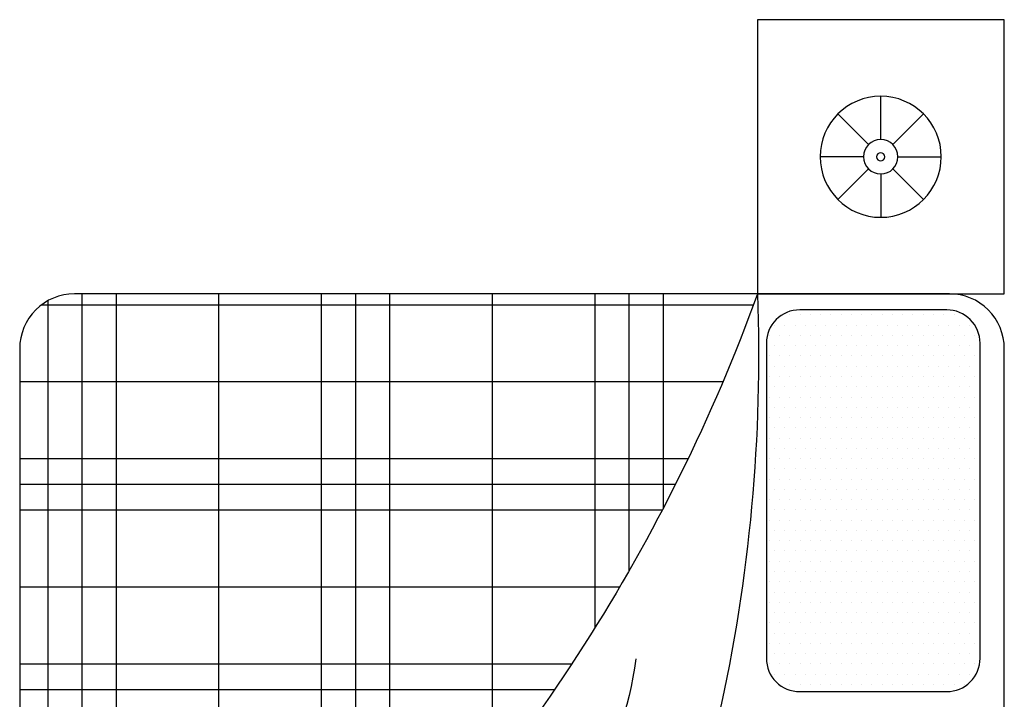
# Model space of a CAD drawing. Units: inches. Extents: x 528 to 2520, y -151 to 1354.
# Tile 12 of 41: x 814 to 869, y 1189 to 1227. Entities that reach past the tile are written whole.
import ezdxf

# ---------------------------------------------------------------- set-up
doc = ezdxf.new("R2010")
doc.units = ezdxf.units.IN
doc.header["$MEASUREMENT"] = 0
doc.layers.add('A-FURN', color=8, linetype='Continuous', lineweight=18)
doc.layers.add('BLOCK', color=6, linetype='Continuous')

# ---------------------------------------------------------------- blocks, each defined once
blk = doc.blocks.new('*X15')
at = {"color": 0}
for p, q in [((276.598, 451.25), (280.51, 451.25)), ((275.455, 450.625), (280.51, 450.625)), ((274.411, 450), (280.51, 450)), ((265.51, 448.125), (267.634, 448.125)), ((271.723, 448.125), (280.51, 448.125)), ((265.51, 446.25), (268.465, 446.25)), ((269.519, 446.25), (280.51, 446.25)), ((265.51, 445.625), (268.531, 445.625)), ((268.866, 445.625), (280.51, 445.625)), ((265.51, 445), (280.51, 445)), ((265.51, 443.125), (280.51, 443.125)), ((265.51, 441.25), (280.51, 441.25)), ((265.51, 440.625), (280.51, 440.625)), ((265.634, 440), (280.386, 440))]:
    blk.add_line(p, q, dxfattribs=at)
blk = doc.blocks.new('*X16')
at = {"color": 0}
for p, q in [((280.312, 439.886), (280.312, 452.896)), ((278.906, 439.482), (278.906, 452.338)), ((277.5, 439.482), (277.5, 451.702)), ((277.031, 439.482), (277.031, 451.471)), ((276.562, 439.482), (276.562, 451.231)), ((275.156, 439.482), (275.156, 450.451)), ((265.781, 439.797), (265.781, 449.511)), ((273.75, 439.482), (273.75, 449.576)), ((266.25, 439.517), (266.25, 449.296)), ((273.281, 439.482), (273.281, 449.261)), ((272.812, 439.482), (272.812, 448.934)), ((267.656, 439.482), (267.656, 448.095)), ((271.406, 439.482), (271.406, 447.876)), ((270, 439.482), (270, 446.689)), ((269.531, 439.482), (269.531, 446.262)), ((269.062, 439.482), (269.062, 445.817))]:
    blk.add_line(p, q, dxfattribs=at)
blk = doc.blocks.new('*X17')
at = {"color": 0}
for p, q in [((273.9375, 457.03125), (273.9375, 457.03125)), ((274.3125, 457.03125), (274.3125, 457.03125)), ((274.6875, 457.03125), (274.6875, 457.03125)), ((275.0625, 457.03125), (275.0625, 457.03125)), ((275.4375, 457.03125), (275.4375, 457.03125)), ((275.8125, 457.03125), (275.8125, 457.03125)), ((276.1875, 457.03125), (276.1875, 457.03125)), ((276.5625, 457.03125), (276.5625, 457.03125)), ((276.9375, 457.03125), (276.9375, 457.03125)), ((277.3125, 457.03125), (277.3125, 457.03125)), ((277.6875, 457.03125), (277.6875, 457.03125)), ((278.0625, 457.03125), (278.0625, 457.03125)), ((278.4375, 457.03125), (278.4375, 457.03125)), ((278.8125, 457.03125), (278.8125, 457.03125)), ((279.1875, 457.03125), (279.1875, 457.03125)), ((279.5625, 457.03125), (279.5625, 457.03125)), ((273.5625, 456.84375), (273.5625, 456.84375)), ((273.75, 456.9375), (273.75, 456.9375)), ((273.9375, 456.84375), (273.9375, 456.84375)), ((274.125, 456.9375), (274.125, 456.9375)), ((274.3125, 456.84375), (274.3125, 456.84375)), ((274.5, 456.9375), (274.5, 456.9375)), ((274.6875, 456.84375), (274.6875, 456.84375)), ((274.875, 456.9375), (274.875, 456.9375)), ((275.0625, 456.84375), (275.0625, 456.84375)), ((275.25, 456.9375), (275.25, 456.9375)), ((275.4375, 456.84375), (275.4375, 456.84375)), ((275.625, 456.9375), (275.625, 456.9375)), ((275.8125, 456.84375), (275.8125, 456.84375)), ((276, 456.9375), (276, 456.9375)), ((276.1875, 456.84375), (276.1875, 456.84375)), ((276.375, 456.9375), (276.375, 456.9375)), ((276.5625, 456.84375), (276.5625, 456.84375)), ((276.75, 456.9375), (276.75, 456.9375)), ((276.9375, 456.84375), (276.9375, 456.84375)), ((277.125, 456.9375), (277.125, 456.9375)), ((277.3125, 456.84375), (277.3125, 456.84375)), ((277.5, 456.9375), (277.5, 456.9375)), ((277.6875, 456.84375), (277.6875, 456.84375)), ((277.875, 456.9375), (277.875, 456.9375)), ((278.0625, 456.84375), (278.0625, 456.84375)), ((278.25, 456.9375), (278.25, 456.9375)), ((278.4375, 456.84375), (278.4375, 456.84375)), ((278.625, 456.9375), (278.625, 456.9375)), ((278.8125, 456.84375), (278.8125, 456.84375)), ((279, 456.9375), (279, 456.9375)), ((279.1875, 456.84375), (279.1875, 456.84375)), ((279.375, 456.9375), (279.375, 456.9375)), ((279.5625, 456.84375), (279.5625, 456.84375)), ((279.75, 456.9375), (279.75, 456.9375)), ((279.9375, 456.84375), (279.9375, 456.84375)), ((273.375, 456.75), (273.375, 456.75)), ((273.75, 456.75), (273.75, 456.75)), ((274.125, 456.75), (274.125, 456.75)), ((274.5, 456.75), (274.5, 456.75)), ((274.875, 456.75), (274.875, 456.75)), ((275.25, 456.75), (275.25, 456.75)), ((275.625, 456.75), (275.625, 456.75)), ((276, 456.75), (276, 456.75)), ((276.375, 456.75), (276.375, 456.75)), ((276.75, 456.75), (276.75, 456.75)), ((277.125, 456.75), (277.125, 456.75)), ((277.5, 456.75), (277.5, 456.75)), ((277.875, 456.75), (277.875, 456.75)), ((278.25, 456.75), (278.25, 456.75)), ((278.625, 456.75), (278.625, 456.75)), ((279, 456.75), (279, 456.75)), ((279.375, 456.75), (279.375, 456.75)), ((279.75, 456.75), (279.75, 456.75)), ((280.125, 456.75), (280.125, 456.75)), ((273.375, 456.5625), (273.375, 456.5625)), ((273.5625, 456.65625), (273.5625, 456.65625)), ((273.75, 456.5625), (273.75, 456.5625)), ((273.9375, 456.65625), (273.9375, 456.65625)), ((274.125, 456.5625), (274.125, 456.5625)), ((274.3125, 456.65625), (274.3125, 456.65625)), ((274.5, 456.5625), (274.5, 456.5625)), ((274.6875, 456.65625), (274.6875, 456.65625)), ((274.875, 456.5625), (274.875, 456.5625)), ((275.0625, 456.65625), (275.0625, 456.65625)), ((275.25, 456.5625), (275.25, 456.5625)), ((275.4375, 456.65625), (275.4375, 456.65625)), ((275.625, 456.5625), (275.625, 456.5625)), ((275.8125, 456.65625), (275.8125, 456.65625)), ((276, 456.5625), (276, 456.5625)), ((276.1875, 456.65625), (276.1875, 456.65625)), ((276.375, 456.5625), (276.375, 456.5625)), ((276.5625, 456.65625), (276.5625, 456.65625)), ((276.75, 456.5625), (276.75, 456.5625)), ((276.9375, 456.65625), (276.9375, 456.65625)), ((277.125, 456.5625), (277.125, 456.5625)), ((277.3125, 456.65625), (277.3125, 456.65625)), ((277.5, 456.5625), (277.5, 456.5625)), ((277.6875, 456.65625), (277.6875, 456.65625)), ((277.875, 456.5625), (277.875, 456.5625)), ((278.0625, 456.65625), (278.0625, 456.65625)), ((278.25, 456.5625), (278.25, 456.5625)), ((278.4375, 456.65625), (278.4375, 456.65625)), ((278.625, 456.5625), (278.625, 456.5625)), ((278.8125, 456.65625), (278.8125, 456.65625)), ((279, 456.5625), (279, 456.5625)), ((279.1875, 456.65625), (279.1875, 456.65625)), ((279.375, 456.5625), (279.375, 456.5625)), ((279.5625, 456.65625), (279.5625, 456.65625)), ((279.75, 456.5625), (279.75, 456.5625)), ((279.9375, 456.65625), (279.9375, 456.65625)), ((280.125, 456.5625), (280.125, 456.5625)), ((273.375, 456.375), (273.375, 456.375)), ((273.5625, 456.46875), (273.5625, 456.46875)), ((273.75, 456.375), (273.75, 456.375)), ((273.9375, 456.46875), (273.9375, 456.46875)), ((274.125, 456.375), (274.125, 456.375)), ((274.3125, 456.46875), (274.3125, 456.46875)), ((274.5, 456.375), (274.5, 456.375)), ((274.6875, 456.46875), (274.6875, 456.46875)), ((274.875, 456.375), (274.875, 456.375)), ((275.0625, 456.46875), (275.0625, 456.46875)), ((275.25, 456.375), (275.25, 456.375)), ((275.4375, 456.46875), (275.4375, 456.46875)), ((275.625, 456.375), (275.625, 456.375)), ((275.8125, 456.46875), (275.8125, 456.46875)), ((276, 456.375), (276, 456.375)), ((276.1875, 456.46875), (276.1875, 456.46875)), ((276.375, 456.375), (276.375, 456.375)), ((276.5625, 456.46875), (276.5625, 456.46875)), ((276.75, 456.375), (276.75, 456.375)), ((276.9375, 456.46875), (276.9375, 456.46875)), ((277.125, 456.375), (277.125, 456.375)), ((277.3125, 456.46875), (277.3125, 456.46875)), ((277.5, 456.375), (277.5, 456.375)), ((277.6875, 456.46875), (277.6875, 456.46875)), ((277.875, 456.375), (277.875, 456.375)), ((278.0625, 456.46875), (278.0625, 456.46875)), ((278.25, 456.375), (278.25, 456.375)), ((278.4375, 456.46875), (278.4375, 456.46875)), ((278.625, 456.375), (278.625, 456.375)), ((278.8125, 456.46875), (278.8125, 456.46875)), ((279, 456.375), (279, 456.375)), ((279.1875, 456.46875), (279.1875, 456.46875)), ((279.375, 456.375), (279.375, 456.375)), ((279.5625, 456.46875), (279.5625, 456.46875)), ((279.75, 456.375), (279.75, 456.375)), ((279.9375, 456.46875), (279.9375, 456.46875)), ((280.125, 456.375), (280.125, 456.375)), ((273.375, 456.1875), (273.375, 456.1875)), ((273.5625, 456.28125), (273.5625, 456.28125)), ((273.75, 456.1875), (273.75, 456.1875)), ((273.9375, 456.28125), (273.9375, 456.28125)), ((274.125, 456.1875), (274.125, 456.1875)), ((274.3125, 456.28125), (274.3125, 456.28125)), ((274.5, 456.1875), (274.5, 456.1875)), ((274.6875, 456.28125), (274.6875, 456.28125)), ((274.875, 456.1875), (274.875, 456.1875)), ((275.0625, 456.28125), (275.0625, 456.28125)), ((275.25, 456.1875), (275.25, 456.1875)), ((275.4375, 456.28125), (275.4375, 456.28125)), ((275.625, 456.1875), (275.625, 456.1875)), ((275.8125, 456.28125), (275.8125, 456.28125)), ((276, 456.1875), (276, 456.1875)), ((276.1875, 456.28125), (276.1875, 456.28125)), ((276.375, 456.1875), (276.375, 456.1875)), ((276.5625, 456.28125), (276.5625, 456.28125)), ((276.75, 456.1875), (276.75, 456.1875)), ((276.9375, 456.28125), (276.9375, 456.28125)), ((277.125, 456.1875), (277.125, 456.1875)), ((277.3125, 456.28125), (277.3125, 456.28125)), ((277.5, 456.1875), (277.5, 456.1875)), ((277.6875, 456.28125), (277.6875, 456.28125)), ((277.875, 456.1875), (277.875, 456.1875)), ((278.0625, 456.28125), (278.0625, 456.28125)), ((278.25, 456.1875), (278.25, 456.1875)), ((278.4375, 456.28125), (278.4375, 456.28125)), ((278.625, 456.1875), (278.625, 456.1875)), ((278.8125, 456.28125), (278.8125, 456.28125)), ((279, 456.1875), (279, 456.1875)), ((279.1875, 456.28125), (279.1875, 456.28125)), ((279.375, 456.1875), (279.375, 456.1875)), ((279.5625, 456.28125), (279.5625, 456.28125)), ((279.75, 456.1875), (279.75, 456.1875)), ((279.9375, 456.28125), (279.9375, 456.28125)), ((280.125, 456.1875), (280.125, 456.1875)), ((273.375, 456), (273.375, 456)), ((273.5625, 456.09375), (273.5625, 456.09375)), ((273.75, 456), (273.75, 456)), ((273.9375, 456.09375), (273.9375, 456.09375)), ((274.125, 456), (274.125, 456)), ((274.3125, 456.09375), (274.3125, 456.09375)), ((274.5, 456), (274.5, 456)), ((274.6875, 456.09375), (274.6875, 456.09375)), ((274.875, 456), (274.875, 456)), ((275.0625, 456.09375), (275.0625, 456.09375)), ((275.25, 456), (275.25, 456)), ((275.4375, 456.09375), (275.4375, 456.09375)), ((275.625, 456), (275.625, 456)), ((275.8125, 456.09375), (275.8125, 456.09375)), ((276, 456), (276, 456)), ((276.1875, 456.09375), (276.1875, 456.09375)), ((276.375, 456), (276.375, 456)), ((276.5625, 456.09375), (276.5625, 456.09375)), ((276.75, 456), (276.75, 456)), ((276.9375, 456.09375), (276.9375, 456.09375)), ((277.125, 456), (277.125, 456)), ((277.3125, 456.09375), (277.3125, 456.09375)), ((277.5, 456), (277.5, 456)), ((277.6875, 456.09375), (277.6875, 456.09375)), ((277.875, 456), (277.875, 456)), ((278.0625, 456.09375), (278.0625, 456.09375)), ((278.25, 456), (278.25, 456)), ((278.4375, 456.09375), (278.4375, 456.09375)), ((278.625, 456), (278.625, 456)), ((278.8125, 456.09375), (278.8125, 456.09375)), ((279, 456), (279, 456)), ((279.1875, 456.09375), (279.1875, 456.09375)), ((279.375, 456), (279.375, 456)), ((279.5625, 456.09375), (279.5625, 456.09375)), ((279.75, 456), (279.75, 456)), ((279.9375, 456.09375), (279.9375, 456.09375)), ((280.125, 456), (280.125, 456)), ((273.375, 455.8125), (273.375, 455.8125)), ((273.5625, 455.90625), (273.5625, 455.90625)), ((273.75, 455.8125), (273.75, 455.8125)), ((273.9375, 455.90625), (273.9375, 455.90625)), ((274.125, 455.8125), (274.125, 455.8125)), ((274.3125, 455.90625), (274.3125, 455.90625)), ((274.5, 455.8125), (274.5, 455.8125)), ((274.6875, 455.90625), (274.6875, 455.90625)), ((274.875, 455.8125), (274.875, 455.8125)), ((275.0625, 455.90625), (275.0625, 455.90625)), ((275.25, 455.8125), (275.25, 455.8125)), ((275.4375, 455.90625), (275.4375, 455.90625)), ((275.625, 455.8125), (275.625, 455.8125)), ((275.8125, 455.90625), (275.8125, 455.90625)), ((276, 455.8125), (276, 455.8125)), ((276.1875, 455.90625), (276.1875, 455.90625)), ((276.375, 455.8125), (276.375, 455.8125)), ((276.5625, 455.90625), (276.5625, 455.90625)), ((276.75, 455.8125), (276.75, 455.8125)), ((276.9375, 455.90625), (276.9375, 455.90625)), ((277.125, 455.8125), (277.125, 455.8125)), ((277.3125, 455.90625), (277.3125, 455.90625)), ((277.5, 455.8125), (277.5, 455.8125)), ((277.6875, 455.90625), (277.6875, 455.90625)), ((277.875, 455.8125), (277.875, 455.8125)), ((278.0625, 455.90625), (278.0625, 455.90625)), ((278.25, 455.8125), (278.25, 455.8125)), ((278.4375, 455.90625), (278.4375, 455.90625)), ((278.625, 455.8125), (278.625, 455.8125)), ((278.8125, 455.90625), (278.8125, 455.90625)), ((279, 455.8125), (279, 455.8125)), ((279.1875, 455.90625), (279.1875, 455.90625)), ((279.375, 455.8125), (279.375, 455.8125)), ((279.5625, 455.90625), (279.5625, 455.90625)), ((279.75, 455.8125), (279.75, 455.8125)), ((279.9375, 455.90625), (279.9375, 455.90625)), ((280.125, 455.8125), (280.125, 455.8125)), ((273.375, 455.625), (273.375, 455.625)), ((273.5625, 455.71875), (273.5625, 455.71875)), ((273.75, 455.625), (273.75, 455.625)), ((273.9375, 455.71875), (273.9375, 455.71875)), ((274.125, 455.625), (274.125, 455.625)), ((274.3125, 455.71875), (274.3125, 455.71875)), ((274.5, 455.625), (274.5, 455.625)), ((274.6875, 455.71875), (274.6875, 455.71875)), ((274.875, 455.625), (274.875, 455.625)), ((275.0625, 455.71875), (275.0625, 455.71875)), ((275.25, 455.625), (275.25, 455.625)), ((275.4375, 455.71875), (275.4375, 455.71875)), ((275.625, 455.625), (275.625, 455.625)), ((275.8125, 455.71875), (275.8125, 455.71875)), ((276, 455.625), (276, 455.625)), ((276.1875, 455.71875), (276.1875, 455.71875)), ((276.375, 455.625), (276.375, 455.625)), ((276.5625, 455.71875), (276.5625, 455.71875)), ((276.75, 455.625), (276.75, 455.625)), ((276.9375, 455.71875), (276.9375, 455.71875)), ((277.125, 455.625), (277.125, 455.625)), ((277.3125, 455.71875), (277.3125, 455.71875)), ((277.5, 455.625), (277.5, 455.625)), ((277.6875, 455.71875), (277.6875, 455.71875)), ((277.875, 455.625), (277.875, 455.625)), ((278.0625, 455.71875), (278.0625, 455.71875)), ((278.25, 455.625), (278.25, 455.625)), ((278.4375, 455.71875), (278.4375, 455.71875)), ((278.625, 455.625), (278.625, 455.625)), ((278.8125, 455.71875), (278.8125, 455.71875)), ((279, 455.625), (279, 455.625)), ((279.1875, 455.71875), (279.1875, 455.71875)), ((279.375, 455.625), (279.375, 455.625)), ((279.5625, 455.71875), (279.5625, 455.71875)), ((279.75, 455.625), (279.75, 455.625)), ((279.9375, 455.71875), (279.9375, 455.71875)), ((280.125, 455.625), (280.125, 455.625)), ((273.375, 455.4375), (273.375, 455.4375)), ((273.5625, 455.53125), (273.5625, 455.53125)), ((273.75, 455.4375), (273.75, 455.4375)), ((273.9375, 455.53125), (273.9375, 455.53125)), ((274.125, 455.4375), (274.125, 455.4375)), ((274.3125, 455.53125), (274.3125, 455.53125)), ((274.5, 455.4375), (274.5, 455.4375)), ((274.6875, 455.53125), (274.6875, 455.53125)), ((274.875, 455.4375), (274.875, 455.4375)), ((275.0625, 455.53125), (275.0625, 455.53125)), ((275.25, 455.4375), (275.25, 455.4375)), ((275.4375, 455.53125), (275.4375, 455.53125)), ((275.625, 455.4375), (275.625, 455.4375)), ((275.8125, 455.53125), (275.8125, 455.53125)), ((276, 455.4375), (276, 455.4375)), ((276.1875, 455.53125), (276.1875, 455.53125)), ((276.375, 455.4375), (276.375, 455.4375)), ((276.5625, 455.53125), (276.5625, 455.53125)), ((276.75, 455.4375), (276.75, 455.4375)), ((276.9375, 455.53125), (276.9375, 455.53125)), ((277.125, 455.4375), (277.125, 455.4375)), ((277.3125, 455.53125), (277.3125, 455.53125)), ((277.5, 455.4375), (277.5, 455.4375)), ((277.6875, 455.53125), (277.6875, 455.53125)), ((277.875, 455.4375), (277.875, 455.4375)), ((278.0625, 455.53125), (278.0625, 455.53125)), ((278.25, 455.4375), (278.25, 455.4375)), ((278.4375, 455.53125), (278.4375, 455.53125)), ((278.625, 455.4375), (278.625, 455.4375)), ((278.8125, 455.53125), (278.8125, 455.53125)), ((279, 455.4375), (279, 455.4375)), ((279.1875, 455.53125), (279.1875, 455.53125)), ((279.375, 455.4375), (279.375, 455.4375)), ((279.5625, 455.53125), (279.5625, 455.53125)), ((279.75, 455.4375), (279.75, 455.4375)), ((279.9375, 455.53125), (279.9375, 455.53125)), ((280.125, 455.4375), (280.125, 455.4375)), ((273.375, 455.25), (273.375, 455.25)), ((273.5625, 455.34375), (273.5625, 455.34375)), ((273.75, 455.25), (273.75, 455.25)), ((273.9375, 455.34375), (273.9375, 455.34375)), ((274.125, 455.25), (274.125, 455.25)), ((274.3125, 455.34375), (274.3125, 455.34375)), ((274.5, 455.25), (274.5, 455.25)), ((274.6875, 455.34375), (274.6875, 455.34375)), ((274.875, 455.25), (274.875, 455.25)), ((275.0625, 455.34375), (275.0625, 455.34375)), ((275.25, 455.25), (275.25, 455.25)), ((275.4375, 455.34375), (275.4375, 455.34375)), ((275.625, 455.25), (275.625, 455.25)), ((275.8125, 455.34375), (275.8125, 455.34375)), ((276, 455.25), (276, 455.25)), ((276.1875, 455.34375), (276.1875, 455.34375)), ((276.375, 455.25), (276.375, 455.25)), ((276.5625, 455.34375), (276.5625, 455.34375)), ((276.75, 455.25), (276.75, 455.25)), ((276.9375, 455.34375), (276.9375, 455.34375)), ((277.125, 455.25), (277.125, 455.25)), ((277.3125, 455.34375), (277.3125, 455.34375)), ((277.5, 455.25), (277.5, 455.25)), ((277.6875, 455.34375), (277.6875, 455.34375)), ((277.875, 455.25), (277.875, 455.25)), ((278.0625, 455.34375), (278.0625, 455.34375)), ((278.25, 455.25), (278.25, 455.25)), ((278.4375, 455.34375), (278.4375, 455.34375)), ((278.625, 455.25), (278.625, 455.25)), ((278.8125, 455.34375), (278.8125, 455.34375)), ((279, 455.25), (279, 455.25)), ((279.1875, 455.34375), (279.1875, 455.34375)), ((279.375, 455.25), (279.375, 455.25)), ((279.5625, 455.34375), (279.5625, 455.34375)), ((279.75, 455.25), (279.75, 455.25)), ((279.9375, 455.34375), (279.9375, 455.34375)), ((280.125, 455.25), (280.125, 455.25)), ((273.375, 455.0625), (273.375, 455.0625)), ((273.5625, 455.15625), (273.5625, 455.15625)), ((273.75, 455.0625), (273.75, 455.0625)), ((273.9375, 455.15625), (273.9375, 455.15625)), ((274.125, 455.0625), (274.125, 455.0625)), ((274.3125, 455.15625), (274.3125, 455.15625)), ((274.5, 455.0625), (274.5, 455.0625)), ((274.6875, 455.15625), (274.6875, 455.15625)), ((274.875, 455.0625), (274.875, 455.0625)), ((275.0625, 455.15625), (275.0625, 455.15625)), ((275.25, 455.0625), (275.25, 455.0625)), ((275.4375, 455.15625), (275.4375, 455.15625)), ((275.625, 455.0625), (275.625, 455.0625)), ((275.8125, 455.15625), (275.8125, 455.15625)), ((276, 455.0625), (276, 455.0625)), ((276.1875, 455.15625), (276.1875, 455.15625)), ((276.375, 455.0625), (276.375, 455.0625)), ((276.5625, 455.15625), (276.5625, 455.15625)), ((276.75, 455.0625), (276.75, 455.0625)), ((276.9375, 455.15625), (276.9375, 455.15625)), ((277.125, 455.0625), (277.125, 455.0625)), ((277.3125, 455.15625), (277.3125, 455.15625)), ((277.5, 455.0625), (277.5, 455.0625)), ((277.6875, 455.15625), (277.6875, 455.15625)), ((277.875, 455.0625), (277.875, 455.0625)), ((278.0625, 455.15625), (278.0625, 455.15625)), ((278.25, 455.0625), (278.25, 455.0625)), ((278.4375, 455.15625), (278.4375, 455.15625)), ((278.625, 455.0625), (278.625, 455.0625)), ((278.8125, 455.15625), (278.8125, 455.15625)), ((279, 455.0625), (279, 455.0625)), ((279.1875, 455.15625), (279.1875, 455.15625)), ((279.375, 455.0625), (279.375, 455.0625)), ((279.5625, 455.15625), (279.5625, 455.15625)), ((279.75, 455.0625), (279.75, 455.0625)), ((279.9375, 455.15625), (279.9375, 455.15625)), ((280.125, 455.0625), (280.125, 455.0625)), ((273.375, 454.875), (273.375, 454.875)), ((273.5625, 454.96875), (273.5625, 454.96875)), ((273.75, 454.875), (273.75, 454.875)), ((273.9375, 454.96875), (273.9375, 454.96875)), ((274.125, 454.875), (274.125, 454.875)), ((274.3125, 454.96875), (274.3125, 454.96875)), ((274.5, 454.875), (274.5, 454.875)), ((274.6875, 454.96875), (274.6875, 454.96875)), ((274.875, 454.875), (274.875, 454.875)), ((275.0625, 454.96875), (275.0625, 454.96875)), ((275.25, 454.875), (275.25, 454.875)), ((275.4375, 454.96875), (275.4375, 454.96875)), ((275.625, 454.875), (275.625, 454.875)), ((275.8125, 454.96875), (275.8125, 454.96875)), ((276, 454.875), (276, 454.875)), ((276.1875, 454.96875), (276.1875, 454.96875)), ((276.375, 454.875), (276.375, 454.875)), ((276.5625, 454.96875), (276.5625, 454.96875)), ((276.75, 454.875), (276.75, 454.875)), ((276.9375, 454.96875), (276.9375, 454.96875)), ((277.125, 454.875), (277.125, 454.875)), ((277.3125, 454.96875), (277.3125, 454.96875)), ((277.5, 454.875), (277.5, 454.875)), ((277.6875, 454.96875), (277.6875, 454.96875)), ((277.875, 454.875), (277.875, 454.875)), ((278.0625, 454.96875), (278.0625, 454.96875)), ((278.25, 454.875), (278.25, 454.875)), ((278.4375, 454.96875), (278.4375, 454.96875)), ((278.625, 454.875), (278.625, 454.875)), ((278.8125, 454.96875), (278.8125, 454.96875)), ((279, 454.875), (279, 454.875)), ((279.1875, 454.96875), (279.1875, 454.96875)), ((279.375, 454.875), (279.375, 454.875)), ((279.5625, 454.96875), (279.5625, 454.96875)), ((279.75, 454.875), (279.75, 454.875)), ((279.9375, 454.96875), (279.9375, 454.96875)), ((280.125, 454.875), (280.125, 454.875)), ((273.375, 454.6875), (273.375, 454.6875)), ((273.5625, 454.78125), (273.5625, 454.78125)), ((273.75, 454.6875), (273.75, 454.6875)), ((273.9375, 454.78125), (273.9375, 454.78125)), ((274.125, 454.6875), (274.125, 454.6875)), ((274.3125, 454.78125), (274.3125, 454.78125)), ((274.5, 454.6875), (274.5, 454.6875)), ((274.6875, 454.78125), (274.6875, 454.78125)), ((274.875, 454.6875), (274.875, 454.6875)), ((275.0625, 454.78125), (275.0625, 454.78125)), ((275.25, 454.6875), (275.25, 454.6875)), ((275.4375, 454.78125), (275.4375, 454.78125)), ((275.625, 454.6875), (275.625, 454.6875)), ((275.8125, 454.78125), (275.8125, 454.78125)), ((276, 454.6875), (276, 454.6875)), ((276.1875, 454.78125), (276.1875, 454.78125)), ((276.375, 454.6875), (276.375, 454.6875)), ((276.5625, 454.78125), (276.5625, 454.78125)), ((276.75, 454.6875), (276.75, 454.6875)), ((276.9375, 454.78125), (276.9375, 454.78125)), ((277.125, 454.6875), (277.125, 454.6875)), ((277.3125, 454.78125), (277.3125, 454.78125)), ((277.5, 454.6875), (277.5, 454.6875)), ((277.6875, 454.78125), (277.6875, 454.78125)), ((277.875, 454.6875), (277.875, 454.6875)), ((278.0625, 454.78125), (278.0625, 454.78125)), ((278.25, 454.6875), (278.25, 454.6875)), ((278.4375, 454.78125), (278.4375, 454.78125)), ((278.625, 454.6875), (278.625, 454.6875)), ((278.8125, 454.78125), (278.8125, 454.78125)), ((279, 454.6875), (279, 454.6875)), ((279.1875, 454.78125), (279.1875, 454.78125)), ((279.375, 454.6875), (279.375, 454.6875)), ((279.5625, 454.78125), (279.5625, 454.78125)), ((279.75, 454.6875), (279.75, 454.6875)), ((279.9375, 454.78125), (279.9375, 454.78125)), ((280.125, 454.6875), (280.125, 454.6875)), ((273.5625, 454.59375), (273.5625, 454.59375)), ((273.9375, 454.59375), (273.9375, 454.59375)), ((274.3125, 454.59375), (274.3125, 454.59375)), ((274.6875, 454.59375), (274.6875, 454.59375)), ((275.0625, 454.59375), (275.0625, 454.59375)), ((275.4375, 454.59375), (275.4375, 454.59375)), ((275.8125, 454.59375), (275.8125, 454.59375)), ((276.1875, 454.59375), (276.1875, 454.59375)), ((276.5625, 454.59375), (276.5625, 454.59375)), ((276.9375, 454.59375), (276.9375, 454.59375)), ((277.3125, 454.59375), (277.3125, 454.59375)), ((277.6875, 454.59375), (277.6875, 454.59375)), ((278.0625, 454.59375), (278.0625, 454.59375)), ((278.4375, 454.59375), (278.4375, 454.59375)), ((278.8125, 454.59375), (278.8125, 454.59375)), ((279.1875, 454.59375), (279.1875, 454.59375)), ((279.5625, 454.59375), (279.5625, 454.59375)), ((279.9375, 454.59375), (279.9375, 454.59375)), ((273.375, 454.5), (273.375, 454.5)), ((273.5625, 454.40625), (273.5625, 454.40625)), ((273.75, 454.5), (273.75, 454.5)), ((273.9375, 454.40625), (273.9375, 454.40625)), ((274.125, 454.5), (274.125, 454.5)), ((274.3125, 454.40625), (274.3125, 454.40625)), ((274.5, 454.5), (274.5, 454.5)), ((274.6875, 454.40625), (274.6875, 454.40625)), ((274.875, 454.5), (274.875, 454.5)), ((275.0625, 454.40625), (275.0625, 454.40625)), ((275.25, 454.5), (275.25, 454.5)), ((275.4375, 454.40625), (275.4375, 454.40625)), ((275.625, 454.5), (275.625, 454.5)), ((275.8125, 454.40625), (275.8125, 454.40625)), ((276, 454.5), (276, 454.5)), ((276.1875, 454.40625), (276.1875, 454.40625)), ((276.375, 454.5), (276.375, 454.5)), ((276.5625, 454.40625), (276.5625, 454.40625)), ((276.75, 454.5), (276.75, 454.5)), ((276.9375, 454.40625), (276.9375, 454.40625)), ((277.125, 454.5), (277.125, 454.5)), ((277.3125, 454.40625), (277.3125, 454.40625)), ((277.5, 454.5), (277.5, 454.5)), ((277.6875, 454.40625), (277.6875, 454.40625)), ((277.875, 454.5), (277.875, 454.5)), ((278.0625, 454.40625), (278.0625, 454.40625)), ((278.25, 454.5), (278.25, 454.5)), ((278.4375, 454.40625), (278.4375, 454.40625)), ((278.625, 454.5), (278.625, 454.5)), ((278.8125, 454.40625), (278.8125, 454.40625)), ((279, 454.5), (279, 454.5)), ((279.1875, 454.40625), (279.1875, 454.40625)), ((279.375, 454.5), (279.375, 454.5)), ((279.5625, 454.40625), (279.5625, 454.40625)), ((279.75, 454.5), (279.75, 454.5)), ((279.9375, 454.40625), (279.9375, 454.40625)), ((280.125, 454.5), (280.125, 454.5)), ((273.375, 454.3125), (273.375, 454.3125)), ((273.5625, 454.21875), (273.5625, 454.21875)), ((273.75, 454.3125), (273.75, 454.3125)), ((273.9375, 454.21875), (273.9375, 454.21875)), ((274.125, 454.3125), (274.125, 454.3125)), ((274.3125, 454.21875), (274.3125, 454.21875)), ((274.5, 454.3125), (274.5, 454.3125)), ((274.6875, 454.21875), (274.6875, 454.21875)), ((274.875, 454.3125), (274.875, 454.3125)), ((275.0625, 454.21875), (275.0625, 454.21875)), ((275.25, 454.3125), (275.25, 454.3125)), ((275.4375, 454.21875), (275.4375, 454.21875)), ((275.625, 454.3125), (275.625, 454.3125)), ((275.8125, 454.21875), (275.8125, 454.21875)), ((276, 454.3125), (276, 454.3125)), ((276.1875, 454.21875), (276.1875, 454.21875)), ((276.375, 454.3125), (276.375, 454.3125)), ((276.5625, 454.21875), (276.5625, 454.21875)), ((276.75, 454.3125), (276.75, 454.3125)), ((276.9375, 454.21875), (276.9375, 454.21875)), ((277.125, 454.3125), (277.125, 454.3125)), ((277.3125, 454.21875), (277.3125, 454.21875)), ((277.5, 454.3125), (277.5, 454.3125)), ((277.6875, 454.21875), (277.6875, 454.21875)), ((277.875, 454.3125), (277.875, 454.3125)), ((278.0625, 454.21875), (278.0625, 454.21875)), ((278.25, 454.3125), (278.25, 454.3125)), ((278.4375, 454.21875), (278.4375, 454.21875)), ((278.625, 454.3125), (278.625, 454.3125)), ((278.8125, 454.21875), (278.8125, 454.21875)), ((279, 454.3125), (279, 454.3125)), ((279.1875, 454.21875), (279.1875, 454.21875)), ((279.375, 454.3125), (279.375, 454.3125)), ((279.5625, 454.21875), (279.5625, 454.21875)), ((279.75, 454.3125), (279.75, 454.3125)), ((279.9375, 454.21875), (279.9375, 454.21875)), ((280.125, 454.3125), (280.125, 454.3125)), ((273.375, 454.125), (273.375, 454.125)), ((273.5625, 454.03125), (273.5625, 454.03125)), ((273.75, 454.125), (273.75, 454.125)), ((273.9375, 454.03125), (273.9375, 454.03125)), ((274.125, 454.125), (274.125, 454.125)), ((274.3125, 454.03125), (274.3125, 454.03125)), ((274.5, 454.125), (274.5, 454.125)), ((274.6875, 454.03125), (274.6875, 454.03125)), ((274.875, 454.125), (274.875, 454.125)), ((275.0625, 454.03125), (275.0625, 454.03125)), ((275.25, 454.125), (275.25, 454.125)), ((275.4375, 454.03125), (275.4375, 454.03125)), ((275.625, 454.125), (275.625, 454.125)), ((275.8125, 454.03125), (275.8125, 454.03125)), ((276, 454.125), (276, 454.125)), ((276.1875, 454.03125), (276.1875, 454.03125)), ((276.375, 454.125), (276.375, 454.125)), ((276.5625, 454.03125), (276.5625, 454.03125)), ((276.75, 454.125), (276.75, 454.125)), ((276.9375, 454.03125), (276.9375, 454.03125)), ((277.125, 454.125), (277.125, 454.125)), ((277.3125, 454.03125), (277.3125, 454.03125)), ((277.5, 454.125), (277.5, 454.125)), ((277.6875, 454.03125), (277.6875, 454.03125)), ((277.875, 454.125), (277.875, 454.125)), ((278.0625, 454.03125), (278.0625, 454.03125)), ((278.25, 454.125), (278.25, 454.125)), ((278.4375, 454.03125), (278.4375, 454.03125)), ((278.625, 454.125), (278.625, 454.125)), ((278.8125, 454.03125), (278.8125, 454.03125)), ((279, 454.125), (279, 454.125)), ((279.1875, 454.03125), (279.1875, 454.03125)), ((279.375, 454.125), (279.375, 454.125)), ((279.5625, 454.03125), (279.5625, 454.03125)), ((279.75, 454.125), (279.75, 454.125)), ((279.9375, 454.03125), (279.9375, 454.03125)), ((280.125, 454.125), (280.125, 454.125)), ((273.375, 453.9375), (273.375, 453.9375)), ((273.5625, 453.84375), (273.5625, 453.84375)), ((273.75, 453.9375), (273.75, 453.9375)), ((273.9375, 453.84375), (273.9375, 453.84375)), ((274.125, 453.9375), (274.125, 453.9375)), ((274.3125, 453.84375), (274.3125, 453.84375)), ((274.5, 453.9375), (274.5, 453.9375)), ((274.6875, 453.84375), (274.6875, 453.84375)), ((274.875, 453.9375), (274.875, 453.9375)), ((275.0625, 453.84375), (275.0625, 453.84375)), ((275.25, 453.9375), (275.25, 453.9375)), ((275.4375, 453.84375), (275.4375, 453.84375)), ((275.625, 453.9375), (275.625, 453.9375)), ((275.8125, 453.84375), (275.8125, 453.84375)), ((276, 453.9375), (276, 453.9375)), ((276.1875, 453.84375), (276.1875, 453.84375)), ((276.375, 453.9375), (276.375, 453.9375)), ((276.5625, 453.84375), (276.5625, 453.84375)), ((276.75, 453.9375), (276.75, 453.9375)), ((276.9375, 453.84375), (276.9375, 453.84375)), ((277.125, 453.9375), (277.125, 453.9375)), ((277.3125, 453.84375), (277.3125, 453.84375)), ((277.5, 453.9375), (277.5, 453.9375)), ((277.6875, 453.84375), (277.6875, 453.84375)), ((277.875, 453.9375), (277.875, 453.9375)), ((278.0625, 453.84375), (278.0625, 453.84375)), ((278.25, 453.9375), (278.25, 453.9375)), ((278.4375, 453.84375), (278.4375, 453.84375)), ((278.625, 453.9375), (278.625, 453.9375)), ((278.8125, 453.84375), (278.8125, 453.84375)), ((279, 453.9375), (279, 453.9375)), ((279.1875, 453.84375), (279.1875, 453.84375)), ((279.375, 453.9375), (279.375, 453.9375)), ((279.5625, 453.84375), (279.5625, 453.84375)), ((279.75, 453.9375), (279.75, 453.9375)), ((279.9375, 453.84375), (279.9375, 453.84375)), ((280.125, 453.9375), (280.125, 453.9375)), ((273.375, 453.75), (273.375, 453.75)), ((273.5625, 453.65625), (273.5625, 453.65625)), ((273.75, 453.75), (273.75, 453.75)), ((273.9375, 453.65625), (273.9375, 453.65625)), ((274.125, 453.75), (274.125, 453.75)), ((274.3125, 453.65625), (274.3125, 453.65625)), ((274.5, 453.75), (274.5, 453.75)), ((274.6875, 453.65625), (274.6875, 453.65625)), ((274.875, 453.75), (274.875, 453.75)), ((275.0625, 453.65625), (275.0625, 453.65625)), ((275.25, 453.75), (275.25, 453.75)), ((275.4375, 453.65625), (275.4375, 453.65625)), ((275.625, 453.75), (275.625, 453.75)), ((275.8125, 453.65625), (275.8125, 453.65625)), ((276, 453.75), (276, 453.75)), ((276.1875, 453.65625), (276.1875, 453.65625)), ((276.375, 453.75), (276.375, 453.75)), ((276.5625, 453.65625), (276.5625, 453.65625)), ((276.75, 453.75), (276.75, 453.75)), ((276.9375, 453.65625), (276.9375, 453.65625)), ((277.125, 453.75), (277.125, 453.75)), ((277.3125, 453.65625), (277.3125, 453.65625)), ((277.5, 453.75), (277.5, 453.75)), ((277.6875, 453.65625), (277.6875, 453.65625)), ((277.875, 453.75), (277.875, 453.75)), ((278.0625, 453.65625), (278.0625, 453.65625)), ((278.25, 453.75), (278.25, 453.75)), ((278.4375, 453.65625), (278.4375, 453.65625)), ((278.625, 453.75), (278.625, 453.75)), ((278.8125, 453.65625), (278.8125, 453.65625)), ((279, 453.75), (279, 453.75)), ((279.1875, 453.65625), (279.1875, 453.65625)), ((279.375, 453.75), (279.375, 453.75)), ((279.5625, 453.65625), (279.5625, 453.65625)), ((279.75, 453.75), (279.75, 453.75)), ((279.9375, 453.65625), (279.9375, 453.65625)), ((280.125, 453.75), (280.125, 453.75)), ((273.375, 453.5625), (273.375, 453.5625)), ((273.5625, 453.46875), (273.5625, 453.46875)), ((273.75, 453.5625), (273.75, 453.5625)), ((273.9375, 453.46875), (273.9375, 453.46875)), ((274.125, 453.5625), (274.125, 453.5625)), ((274.3125, 453.46875), (274.3125, 453.46875)), ((274.5, 453.5625), (274.5, 453.5625)), ((274.6875, 453.46875), (274.6875, 453.46875)), ((274.875, 453.5625), (274.875, 453.5625)), ((275.0625, 453.46875), (275.0625, 453.46875)), ((275.25, 453.5625), (275.25, 453.5625)), ((275.4375, 453.46875), (275.4375, 453.46875)), ((275.625, 453.5625), (275.625, 453.5625)), ((275.8125, 453.46875), (275.8125, 453.46875)), ((276, 453.5625), (276, 453.5625)), ((276.1875, 453.46875), (276.1875, 453.46875)), ((276.375, 453.5625), (276.375, 453.5625)), ((276.5625, 453.46875), (276.5625, 453.46875)), ((276.75, 453.5625), (276.75, 453.5625)), ((276.9375, 453.46875), (276.9375, 453.46875)), ((277.125, 453.5625), (277.125, 453.5625)), ((277.3125, 453.46875), (277.3125, 453.46875)), ((277.5, 453.5625), (277.5, 453.5625)), ((277.6875, 453.46875), (277.6875, 453.46875)), ((277.875, 453.5625), (277.875, 453.5625)), ((278.0625, 453.46875), (278.0625, 453.46875)), ((278.25, 453.5625), (278.25, 453.5625)), ((278.4375, 453.46875), (278.4375, 453.46875)), ((278.625, 453.5625), (278.625, 453.5625)), ((278.8125, 453.46875), (278.8125, 453.46875)), ((279, 453.5625), (279, 453.5625)), ((279.1875, 453.46875), (279.1875, 453.46875)), ((279.375, 453.5625), (279.375, 453.5625)), ((279.5625, 453.46875), (279.5625, 453.46875)), ((279.75, 453.5625), (279.75, 453.5625)), ((279.9375, 453.46875), (279.9375, 453.46875)), ((280.125, 453.5625), (280.125, 453.5625)), ((273.375, 453.375), (273.375, 453.375)), ((273.5625, 453.28125), (273.5625, 453.28125)), ((273.75, 453.375), (273.75, 453.375)), ((273.9375, 453.28125), (273.9375, 453.28125)), ((274.125, 453.375), (274.125, 453.375)), ((274.3125, 453.28125), (274.3125, 453.28125)), ((274.5, 453.375), (274.5, 453.375)), ((274.6875, 453.28125), (274.6875, 453.28125)), ((274.875, 453.375), (274.875, 453.375)), ((275.0625, 453.28125), (275.0625, 453.28125)), ((275.25, 453.375), (275.25, 453.375)), ((275.4375, 453.28125), (275.4375, 453.28125)), ((275.625, 453.375), (275.625, 453.375)), ((275.8125, 453.28125), (275.8125, 453.28125)), ((276, 453.375), (276, 453.375)), ((276.1875, 453.28125), (276.1875, 453.28125)), ((276.375, 453.375), (276.375, 453.375)), ((276.5625, 453.28125), (276.5625, 453.28125)), ((276.75, 453.375), (276.75, 453.375)), ((276.9375, 453.28125), (276.9375, 453.28125)), ((277.125, 453.375), (277.125, 453.375)), ((277.3125, 453.28125), (277.3125, 453.28125)), ((277.5, 453.375), (277.5, 453.375)), ((277.6875, 453.28125), (277.6875, 453.28125)), ((277.875, 453.375), (277.875, 453.375)), ((278.0625, 453.28125), (278.0625, 453.28125)), ((278.25, 453.375), (278.25, 453.375)), ((278.4375, 453.28125), (278.4375, 453.28125)), ((278.625, 453.375), (278.625, 453.375)), ((278.8125, 453.28125), (278.8125, 453.28125)), ((279, 453.375), (279, 453.375)), ((279.1875, 453.28125), (279.1875, 453.28125)), ((279.375, 453.375), (279.375, 453.375)), ((279.5625, 453.28125), (279.5625, 453.28125)), ((279.75, 453.375), (279.75, 453.375)), ((279.9375, 453.28125), (279.9375, 453.28125)), ((273.75, 453.1875), (273.75, 453.1875)), ((274.125, 453.1875), (274.125, 453.1875)), ((274.5, 453.1875), (274.5, 453.1875)), ((274.875, 453.1875), (274.875, 453.1875)), ((275.25, 453.1875), (275.25, 453.1875)), ((275.625, 453.1875), (275.625, 453.1875)), ((276, 453.1875), (276, 453.1875)), ((276.375, 453.1875), (276.375, 453.1875)), ((276.75, 453.1875), (276.75, 453.1875)), ((277.125, 453.1875), (277.125, 453.1875)), ((277.5, 453.1875), (277.5, 453.1875)), ((277.875, 453.1875), (277.875, 453.1875)), ((278.25, 453.1875), (278.25, 453.1875)), ((278.625, 453.1875), (278.625, 453.1875)), ((279, 453.1875), (279, 453.1875)), ((279.375, 453.1875), (279.375, 453.1875)), ((279.75, 453.1875), (279.75, 453.1875))]:
    blk.add_line(p, q, dxfattribs=at)
blk = doc.blocks.new('A$C52E67D0D')
at = {"layer": 'BLOCK'}
for p, q in [((2251.5, 1605.5), (2251.5, 1684.7)), ((2229.3, 1596.3), (2173.3, 1652.3)), ((2273.7, 1596.3), (2329.7, 1652.3)), ((2220.1, 1574.1), (2140.9, 1574.1)), ((2282.9, 1574.1), (2362.1, 1574.1)), ((2229.3, 1551.9), (2173.3, 1495.9)), ((2273.7, 1551.9), (2329.7, 1495.9)), ((2251.5, 1542.8), (2251.5, 1463.5))]:
    blk.add_line(p, q, dxfattribs=at)
for points in [[(1901, 0), (601, 0, -0.414214), (501, 100), (501, 1700, -0.414214), (601, 1800), (1901, 1800, -0.414214), (2001, 1700), (2001, 100, -0.414214)], [(1911, 1365.1), (1335, 1365.1, -0.414214), (1274.2, 1425.9), (1274.2, 1694.8, -0.414214), (1335, 1755.7), (1911, 1755.7, -0.414214), (1971.8, 1694.8), (1971.8, 1425.9, -0.414214)]]:
    blk.add_lwpolyline(points, format="xyb", close=True, dxfattribs=at)
blk.add_lwpolyline([(2001, 1348.6), (2001, 1799.6), (2502, 1799.6), (2502, 1348.6)], close=True, dxfattribs=at)
for radius in [110.6, 31.4, 7.46]:
    blk.add_circle((2251.5, 1574.1), radius, dxfattribs=at)
for centre, radius, start, end in [((1888.6, -1664.5), 3015.3, 87.8642, 117.4001), ((3101, -1685.8), 3227.7, 109.926, 135.3977), ((1410.8, 520.2), 610.8, 97.2157, 147.6656)]:
    blk.add_arc(centre, radius, start, end, dxfattribs=at)
at = {"layer": 'BLOCK', "xscale": 100, "yscale": 100, "zscale": 100}
for name in ['*X17', '*X16', '*X15']:
    blk.add_blockref(name, (-26050, -43948.2), dxfattribs=at)

msp = doc.modelspace()

# ---------------------------------------------------------------- block references
at = {"layer": 'A-FURN', "xscale": -0.0306954436450662, "yscale": 0.0306954436450662, "zscale": 0.0306954436450662, "rotation": 270}
msp.add_blockref('A$C52E67D0D', (813.801, 1150.631), dxfattribs=at)

doc.saveas('drawing.dxf')
